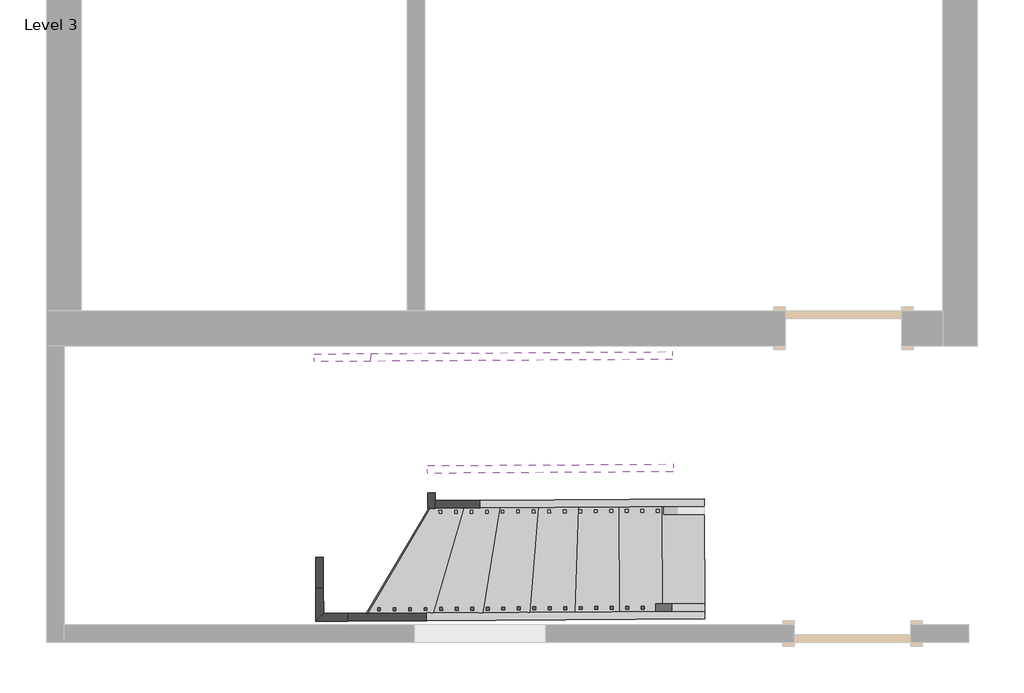
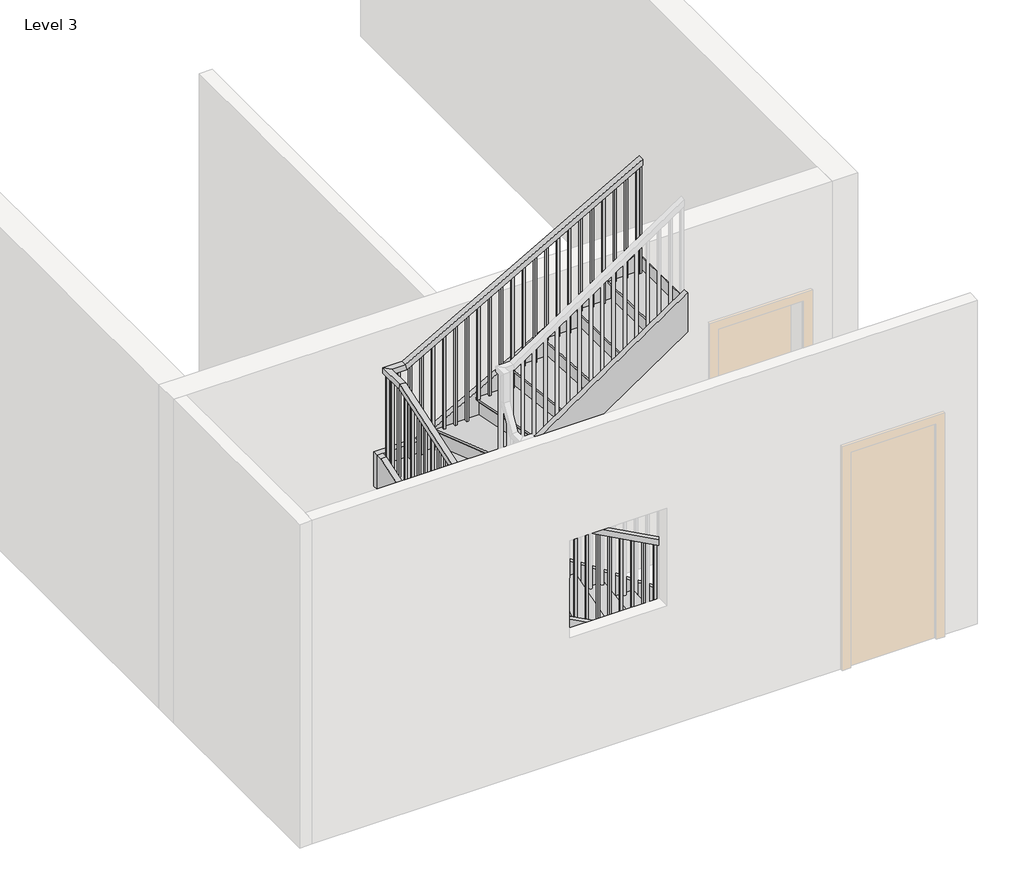
# One storey, part 2 of 2: 9 members, 1 railing, 1 stair flight.
"""IFC4 building model written with IfcOpenShell, lengths in millimetres."""

from ifc_helpers import new_model, si_unit, frame, origin, place, context, project, spatial, polyline, outline, extrude, faceted_brep, transform, mapped, element, save
from components import stair_flight_20cd7bae

model = new_model("IFC4")

# Units and contexts
model_context = context("Model", 3, world=origin())
ifc_project = project(units=[si_unit("LENGTHUNIT", "METRE", prefix="MILLI")], contexts=[model_context])

# Site, building, storey
site = spatial("IfcSite", under=ifc_project)
building = spatial("IfcBuilding", under=site)
storey = spatial("IfcBuildingStorey", under=building, Name="Level 3", Elevation=3200.4)

# Members
placement = place(None, origin())
element("IfcMember", 1, ObjectType="Stringer - 2\" Width", at=placement, inside=storey, context=model_context, shape_type="SweptSolid", body=[
    extrude(outline(polyline([(-106.4787477, -199.0602913), (0.0, 0.0), (2650.4216713, 0.0), (2487.3820108, -304.8), (91.199922, -304.8), (-106.4787477, -199.0602913)])), frame((-116.1777511, -4276.2080688, 3426.1492487), z_axis=(-0.006129891180436153, 0.9999812120405643, 0.0), x_axis=(-0.8817595296628616, -0.005405191516664865, 0.47166822635555733)), (0.0, 0.0, 1.0), 50.8),
])
element("IfcMember", 2, ObjectType="Stringer - 2\" Width", at=placement, inside=storey, context=model_context, shape_type="SweptSolid", body=[
    extrude(outline(polyline([(-2453.5237158, -4239.7350599), (-2453.2123174, -4290.5341055), (-2663.1420684, -4291.8209762), (-2612.6544213, -4240.7105322), (-2453.5237158, -4239.7350599)])), frame((0.0, 0.0, 4330.6029558), z_axis=(0.0, 0.0, 1.0), x_axis=(1.0, 0.0, 0.0)), (0.0, 0.0, 1.0), 345.6659817),
])
element("IfcMember", 3, ObjectType="Stringer - 2\" Width", at=placement, inside=storey, context=model_context, shape_type="SweptSolid", body=[
    extrude(outline(polyline([(-2612.6544213, -4240.7105322), (-2663.1420684, -4291.8209762), (-2664.4731567, -4074.6779247), (-2613.6741111, -4074.3665263), (-2612.6544213, -4240.7105322)])), frame((0.0, 0.0, 4330.6029558), z_axis=(0.0, 0.0, 1.0), x_axis=(1.0, 0.0, 0.0)), (0.0, 0.0, 1.0), 345.6659817),
])
element("IfcMember", 4, ObjectType="Stringer - 2\" Width", at=placement, inside=storey, context=model_context, shape_type="SweptSolid", body=[
    extrude(outline(polyline([(-112.9595567, -326.688092), (0.0, 0.0), (1516.7940002, 1e-07), (1565.1210838, -16.7101466), (1457.9394259, -326.6880919), (-112.9595567, -326.688092)])), frame((-2664.4731567, -4074.6779247, 4676.2689375), z_axis=(0.9999812120405643, 0.006129891180436426, 0.0), x_axis=(-0.005793345483301552, 0.9450798501367781, 0.3267881791215163)), (0.0, 0.0, 1.0), 50.8),
])
element("IfcMember", 5, ObjectType="Stringer - 2\" Width", at=placement, inside=storey, context=model_context, shape_type="SweptSolid", body=[
    extrude(outline(polyline([(-111.800968, -163.7049666), (0.0, 0.0), (2130.8093531, 0.0), (1922.648686, -304.8000001), (94.7979387, -304.8000001), (-111.800968, -163.7049666)])), frame((-120.6930289, -3539.621908, 3398.6391801), z_axis=(-0.006129891180436334, 0.9999812120405644, 0.0), x_axis=(-0.8257797012408891, -0.005062034812924603, 0.5639700885880925)), (0.0, 0.0, 1.0), 50.8),
])
element("IfcMember", 6, ObjectType="Stringer - 2\" Width", at=placement, inside=storey, context=model_context, shape_type="SweptSolid", body=[
    extrude(outline(polyline([(-476.3090819, -288.3824073), (0.0, 0.0), (441.380003, 0.0), (-62.0453256, -304.8), (-466.3690133, -304.8), (-476.3090819, -288.3824073)])), frame((-1931.0711854, -3550.7195376, 4822.7542381), z_axis=(0.9999812120405644, 0.006129891180436036, 0.0), x_axis=(-0.00317479975135555, 0.5179113315223286, 0.8554284150806002)), (0.0, 0.0, 1.0), 50.8),
])
element("IfcMember", 7, ObjectType="Stringer - 2\" Width", at=placement, inside=storey, context=model_context, shape_type="SweptSolid", body=[
    extrude(outline(polyline([(205.0123517, -304.8), (0.0, 0.0), (1938.1040339, 0.0), (2143.1163855, -304.8), (205.0123517, -304.8)])), frame((-1932.4724786, -3322.1238325, 4867.3006308), z_axis=(-0.006129891180436482, 0.9999812120405644, 0.0), x_axis=(0.8297505463599371, 0.005086376118722323, 0.5581112430271987)), (0.0, 0.0, 1.0), 50.8),
])
element("IfcMember", 8, ObjectType="Stringer - 2\" Width", at=placement, inside=storey, context=model_context, shape_type="SweptSolid", body=[
    extrude(outline(polyline([(-2673.5739172, -2590.0529496), (-2673.8853157, -2539.253904), (-2303.2697085, -2536.982028), (-2302.9583101, -2587.7810735), (-2673.5739172, -2590.0529496)])), frame((0.0, 0.0, 4849.4329153), z_axis=(0.0, 0.0, 1.0), x_axis=(1.0, 0.0, 0.0)), (0.0, 0.0, 1.0), 322.5063717),
])
element("IfcMember", 9, ObjectType="Stringer - 2\" Width", at=placement, inside=storey, context=model_context, shape_type="SweptSolid", body=[
    extrude(outline(polyline([(155.3220552, -282.6400873), (0.0, 0.0), (2252.6037587, 1e-07), (2407.9258139, -282.6400872), (155.3220552, -282.6400873)])), frame((-2302.9583101, -2587.7810735, 4849.4329153), z_axis=(-0.00612989118043627, 0.9999812120405644, 0.0), x_axis=(0.8763695910030254, 0.005372151158450033, 0.48160926066378834)), (0.0, 0.0, 1.0), 50.8),
])

# Railing
element("IfcRailing", 10, ObjectType="Handrail - Rectangular", at=placement, inside=storey, context=model_context, shape_type="SolidModel", body=[
    faceted_brep([(-116.4891496, -4225.4090232, 4284.1333333), (-116.4891496, -4225.4090232, 4226.3022634), (-116.800548, -4174.6099776, 4226.3022634), (-116.800548, -4174.6099776, 4284.1333333), (-2474.2717021, -4239.8622452, 5566.8653479), (-2487.1954725, -4239.941468, 5516.0653479), (-2487.506871, -4189.1424224, 5516.0653479), (-2474.5831006, -4189.0631997, 5566.8653479), (-2612.6544213, -4240.7105322, 5566.8653479), (-2612.6544213, -4240.7105322, 5516.0653479), (-2562.1667742, -4189.6000881, 5516.0653479), (-2562.1667742, -4189.6000881, 5566.8653479), (-2613.899826, -4037.5452114, 5566.8653479), (-2613.9521428, -4029.010664, 5516.0653479), (-2563.1530973, -4028.6992655, 5516.0653479), (-2563.1007804, -4037.2338129, 5566.8653479), (-2621.180916, -2849.7666717, 5977.5734867), (-2621.2332328, -2841.2321243, 5926.7734867), (-2570.4341872, -2840.9207258, 5926.7734867), (-2570.3818704, -2849.4552732, 5977.5734867), (-2622.7748716, -2589.7415511, 5977.5734867), (-2622.7748716, -2589.7415511, 5926.7734867), (-2571.6644276, -2640.2291982, 5926.7734867), (-2571.6644276, -2640.2291982, 5977.5734867), (-2452.0429693, -2588.6949634, 5977.5734867), (-2438.8245474, -2588.6139344, 5926.7734867), (-2438.513149, -2639.41298, 5926.7734867), (-2451.7315708, -2639.494009, 5977.5734867), (-328.8448754, -2575.6797456, 7162.8), (-328.533477, -2626.4787912, 7162.8), (-328.533477, -2626.4787912, 7104.62112), (-328.8448754, -2575.6797456, 7104.62112)], [[[0, 1, 2, 3]], [[1, 0, 4, 5]], [[2, 1, 5, 6]], [[3, 2, 6, 7]], [[0, 3, 7, 4]], [[5, 4, 8, 9]], [[6, 5, 9, 10]], [[7, 6, 10, 11]], [[4, 7, 11, 8]], [[9, 8, 12, 13]], [[10, 9, 13, 14]], [[11, 10, 14, 15]], [[8, 11, 15, 12]], [[13, 12, 16, 17]], [[14, 13, 17, 18]], [[15, 14, 18, 19]], [[12, 15, 19, 16]], [[17, 16, 20, 21]], [[18, 17, 21, 22]], [[19, 18, 22, 23]], [[16, 19, 23, 20]], [[21, 20, 24, 25]], [[22, 21, 25, 26]], [[23, 22, 26, 27]], [[20, 23, 27, 24]], [[28, 29, 30, 31]], [[25, 24, 28, 31]], [[26, 25, 31, 30]], [[27, 26, 30, 29]], [[24, 27, 29, 28]]]),
    extrude(outline(polyline([(233.9170124, 19.05), (1235.5250403, 19.05), (1235.5250403, 0.0), (223.2829877, 0.0), (233.9170124, 19.05)])), frame((-352.4784362, -2610.7502757, 7314.591707), z_axis=(-0.0061298911804362555, 0.9999812120405644, 0.0), x_axis=(0.0, 0.0, -1.0)), (0.0, 0.0, 1.0), 19.05),
    extrude(outline(polyline([(233.9170123, 19.05), (1178.8102421, 19.05), (1178.8102421, 0.0), (223.2829877, 0.0), (233.9170123, 19.05)])), frame((-454.0765273, -2611.3730726, 7257.8769088), z_axis=(-0.0061298911804362555, 0.9999812120405644, 0.0), x_axis=(0.0, 0.0, -1.0)), (0.0, 0.0, 1.0), 19.05),
    extrude(outline(polyline([(233.9170124, 19.05), (1122.095444, 19.05), (1122.095444, 0.0), (223.2829877, 0.0), (233.9170124, 19.05)])), frame((-555.6746185, -2611.9958696, 7201.1621107), z_axis=(-0.0061298911804362555, 0.9999812120405644, 0.0), x_axis=(0.0, 0.0, -1.0)), (0.0, 0.0, 1.0), 19.05),
    extrude(outline(polyline([(233.9170123, 19.05), (1234.7139792, 19.05), (1234.7139792, 0.0), (223.2829877, 0.0), (233.9170123, 19.05)])), frame((-657.2727096, -2612.6186665, 7144.4473125), z_axis=(-0.0061298911804362555, 0.9999812120405644, 0.0), x_axis=(0.0, 0.0, -1.0)), (0.0, 0.0, 1.0), 19.05),
    extrude(outline(polyline([(233.9170123, 19.05), (1177.999181, 19.05), (1177.999181, 0.0), (223.2829876, 0.0), (233.9170123, 19.05)])), frame((-758.8708008, -2613.2414635, 7087.7325143), z_axis=(-0.0061298911804362555, 0.9999812120405644, 0.0), x_axis=(0.0, 0.0, -1.0)), (0.0, 0.0, 1.0), 19.05),
    extrude(outline(polyline([(233.9170123, 19.05), (1121.2843829, 19.05), (1121.2843829, 0.0), (223.2829877, 0.0), (233.9170123, 19.05)])), frame((-860.4688919, -2613.8642604, 7031.0177162), z_axis=(-0.0061298911804362555, 0.9999812120405644, 0.0), x_axis=(0.0, 0.0, -1.0)), (0.0, 0.0, 1.0), 19.05),
    extrude(outline(polyline([(233.9170123, 19.0499999), (1233.902918, 19.0499999), (1233.902918, 0.0), (223.2829876, 0.0), (233.9170123, 19.0499999)])), frame((-962.0669831, -2614.4870574, 6974.302918), z_axis=(-0.0061298911804362555, 0.9999812120405644, 0.0), x_axis=(0.0, 0.0, -1.0)), (0.0, 0.0, 1.0), 19.05),
    extrude(outline(polyline([(233.9170123, 19.05), (1177.1881199, 19.05), (1177.1881199, 0.0), (223.2829877, 0.0), (233.9170123, 19.05)])), frame((-1063.6650742, -2615.1098543, 6917.5881199), z_axis=(-0.0061298911804362555, 0.9999812120405644, 0.0), x_axis=(0.0, 0.0, -1.0)), (0.0, 0.0, 1.0), 19.05),
    extrude(outline(polyline([(233.9170123, 19.05), (1120.4733217, 19.05), (1120.4733217, 0.0), (223.2829876, 0.0), (233.9170123, 19.05)])), frame((-1165.2631653, -2615.7326513, 6860.8733217), z_axis=(-0.0061298911804362555, 0.9999812120405644, 0.0), x_axis=(0.0, 0.0, -1.0)), (0.0, 0.0, 1.0), 19.05),
    extrude(outline(polyline([(233.9170123, 19.05), (1233.0918569, 19.05), (1233.0918569, 0.0), (223.2829877, 0.0), (233.9170123, 19.05)])), frame((-1266.8612565, -2616.3554482, 6804.1585236), z_axis=(-0.0061298911804362555, 0.9999812120405644, 0.0), x_axis=(0.0, 0.0, -1.0)), (0.0, 0.0, 1.0), 19.05),
    extrude(outline(polyline([(233.9170123, 19.05), (1176.3770587, 19.05), (1176.3770587, 0.0), (223.2829876, 0.0), (233.9170123, 19.05)])), frame((-1368.4593476, -2616.9782451, 6747.4437254), z_axis=(-0.0061298911804362555, 0.9999812120405644, 0.0), x_axis=(0.0, 0.0, -1.0)), (0.0, 0.0, 1.0), 19.05),
    extrude(outline(polyline([(233.9170123, 19.05), (1288.995594, 19.05), (1288.995594, 0.0), (223.2829877, 0.0), (233.9170123, 19.05)])), frame((-1470.0574388, -2617.6010421, 6690.7289273), z_axis=(-0.0061298911804362555, 0.9999812120405644, 0.0), x_axis=(0.0, 0.0, -1.0)), (0.0, 0.0, 1.0), 19.05),
    extrude(outline(polyline([(233.9170123, 19.05), (1232.2807958, 19.05), (1232.2807958, 0.0), (223.2829876, 0.0), (233.9170123, 19.05)])), frame((-1571.6555299, -2618.223839, 6634.0141291), z_axis=(-0.0061298911804362555, 0.9999812120405644, 0.0), x_axis=(0.0, 0.0, -1.0)), (0.0, 0.0, 1.0), 19.05),
    extrude(outline(polyline([(233.9170123, 19.05), (1175.5659977, 19.05), (1175.5659977, 0.0), (223.2829877, 0.0), (233.9170123, 19.05)])), frame((-1673.2536211, -2618.846636, 6577.299331), z_axis=(-0.0061298911804362555, 0.9999812120405644, 0.0), x_axis=(0.0, 0.0, -1.0)), (0.0, 0.0, 1.0), 19.05),
    extrude(outline(polyline([(233.9170123, 19.05), (1118.8511995, 19.05), (1118.8511995, 0.0), (223.2829876, 0.0), (233.9170123, 19.05)])), frame((-1774.8517122, -2619.4694329, 6520.5845328), z_axis=(-0.0061298911804362555, 0.9999812120405644, 0.0), x_axis=(0.0, 0.0, -1.0)), (0.0, 0.0, 1.0), 19.05),
    extrude(outline(polyline([(233.9170123, 19.05), (1231.4697347, 19.05), (1231.4697347, 0.0), (223.2829877, 0.0), (233.9170123, 19.05)])), frame((-1876.4498033, -2620.0922299, 6463.8697347), z_axis=(-0.0061298911804362555, 0.9999812120405644, 0.0), x_axis=(0.0, 0.0, -1.0)), (0.0, 0.0, 1.0), 19.05),
    extrude(outline(polyline([(233.9170123, 19.05), (1174.7549365, 19.05), (1174.7549365, 0.0), (223.2829876, 0.0), (233.9170123, 19.05)])), frame((-1978.0478945, -2620.7150268, 6407.1549365), z_axis=(-0.0061298911804362555, 0.9999812120405644, 0.0), x_axis=(0.0, 0.0, -1.0)), (0.0, 0.0, 1.0), 19.05),
    extrude(outline(polyline([(233.9170124, 19.05), (1118.0401384, 19.05), (1118.0401384, 0.0), (223.2829877, 0.0), (233.9170124, 19.05)])), frame((-2079.6459856, -2621.3378238, 6350.4401384), z_axis=(-0.0061298911804362555, 0.9999812120405644, 0.0), x_axis=(0.0, 0.0, -1.0)), (0.0, 0.0, 1.0), 19.05),
    extrude(outline(polyline([(233.9170123, 19.05), (1230.6586735, 19.05), (1230.6586735, 0.0), (223.2829876, 0.0), (233.9170123, 19.05)])), frame((-2181.2440768, -2621.9606207, 6293.7253402), z_axis=(-0.0061298911804362555, 0.9999812120405644, 0.0), x_axis=(0.0, 0.0, -1.0)), (0.0, 0.0, 1.0), 19.05),
    extrude(outline(polyline([(233.9170124, 19.05), (1173.9438754, 19.05), (1173.9438754, 0.0), (223.2829877, 0.0), (233.9170124, 19.05)])), frame((-2282.8421679, -2622.5834176, 6237.0105421), z_axis=(-0.0061298911804362555, 0.9999812120405644, 0.0), x_axis=(0.0, 0.0, -1.0)), (0.0, 0.0, 1.0), 19.05),
    extrude(outline(polyline([(233.9170123, 19.05), (1117.2290772, 19.05), (1117.2290772, 0.0), (223.2829877, 0.0), (233.9170123, 19.05)])), frame((-2384.4402591, -2623.2062146, 6180.2957439), z_axis=(-0.0061298911804362555, 0.9999812120405644, 0.0), x_axis=(0.0, 0.0, -1.0)), (0.0, 0.0, 1.0), 19.05),
    extrude(outline(polyline([(-2505.2047667, -2604.8961439), (-2486.1551246, -2604.7793694), (-2486.0383502, -2623.8290115), (-2505.0879923, -2623.945786), (-2505.2047667, -2604.8961439)])), frame((0.0, 0.0, 5063.0666667), z_axis=(0.0, 0.0, 1.0), x_axis=(1.0, 0.0, 0.0)), (0.0, 0.0, 1.0), 863.70682),
    extrude(outline(polyline([(-2606.2189857, -2700.7671513), (-2606.3357602, -2681.7175092), (-2587.2861181, -2681.6007347), (-2587.1693436, -2700.6503768), (-2606.2189857, -2700.7671513)])), frame((0.0, 0.0, 5063.0666667), z_axis=(0.0, 0.0, 1.0), x_axis=(1.0, 0.0, 0.0)), (0.0, 0.0, 1.0), 863.70682),
    extrude(outline(polyline([(-2605.5961888, -2802.3652424), (-2605.7129632, -2783.3156003), (-2586.6633211, -2783.1988259), (-2586.5465467, -2802.248468), (-2605.5961888, -2802.3652424)])), frame((0.0, 0.0, 5063.0666667), z_axis=(0.0, 0.0, 1.0), x_axis=(1.0, 0.0, 0.0)), (0.0, 0.0, 1.0), 863.70682),
    extrude(outline(polyline([(225.3065228, 19.0499999), (1243.2088863, 19.0499999), (1243.2088863, 0.0), (231.8934772, 0.0), (225.3065228, 19.0499999)])), frame((-2604.9733918, -2903.9633335, 6136.9422196), z_axis=(0.9999812120405643, 0.0061298911804362685, 0.0), x_axis=(0.0, 0.0, -1.0)), (0.0, 0.0, 1.0), 19.05),
    extrude(outline(polyline([(225.3065229, 19.05), (1208.078463, 19.05), (1208.078463, 0.0), (231.8934772, 0.0), (225.3065229, 19.05)])), frame((-2604.3505949, -3005.5614247, 6101.8117963), z_axis=(0.9999812120405643, 0.0061298911804362685, 0.0), x_axis=(0.0, 0.0, -1.0)), (0.0, 0.0, 1.0), 19.05),
    extrude(outline(polyline([(225.3065228, 19.05), (1172.9480396, 19.05), (1172.9480396, 0.0), (231.8934772, 0.0), (225.3065228, 19.05)])), frame((-2603.727798, -3107.1595158, 6066.6813729), z_axis=(0.9999812120405643, 0.0061298911804362685, 0.0), x_axis=(0.0, 0.0, -1.0)), (0.0, 0.0, 1.0), 19.05),
    extrude(outline(polyline([(225.3065228, 19.05), (1137.8176163, 19.05), (1137.8176163, 0.0), (231.8934772, 0.0), (225.3065228, 19.05)])), frame((-2603.105001, -3208.757607, 6031.5509496), z_axis=(0.9999812120405643, 0.0061298911804362685, 0.0), x_axis=(0.0, 0.0, -1.0)), (0.0, 0.0, 1.0), 19.05),
    extrude(outline(polyline([(225.3065228, 19.05), (1102.687193, 19.05), (1102.687193, 0.0), (231.8934772, 0.0), (225.3065228, 19.05)])), frame((-2602.4822041, -3310.3556981, 5996.4205263), z_axis=(0.9999812120405643, 0.0061298911804362685, 0.0), x_axis=(0.0, 0.0, -1.0)), (0.0, 0.0, 1.0), 19.05),
    extrude(outline(polyline([(225.3065228, 19.05), (1236.890103, 19.05), (1236.890103, 0.0), (231.8934772, 0.0), (225.3065228, 19.05)])), frame((-2601.8594071, -3411.9537893, 5961.290103), z_axis=(0.9999812120405643, 0.0061298911804362685, 0.0), x_axis=(0.0, 0.0, -1.0)), (0.0, 0.0, 1.0), 19.05),
    extrude(outline(polyline([(225.3065229, 19.05), (1201.7596797, 19.05), (1201.7596797, 0.0), (231.8934772, 0.0), (225.3065229, 19.05)])), frame((-2601.2366102, -3513.5518804, 5926.1596797), z_axis=(0.9999812120405643, 0.0061298911804362685, 0.0), x_axis=(0.0, 0.0, -1.0)), (0.0, 0.0, 1.0), 19.05),
    extrude(outline(polyline([(225.3065228, 19.0499999), (1166.6292563, 19.0499999), (1166.6292563, 0.0), (231.8934772, 0.0), (225.3065228, 19.0499999)])), frame((-2600.6138132, -3615.1499715, 5891.0292563), z_axis=(0.9999812120405643, 0.0061298911804362685, 0.0), x_axis=(0.0, 0.0, -1.0)), (0.0, 0.0, 1.0), 19.05),
    extrude(outline(polyline([(225.3065228, 19.05), (1131.498833, 19.05), (1131.498833, 0.0), (231.8934772, 0.0), (225.3065228, 19.05)])), frame((-2599.9910163, -3716.7480627, 5855.898833), z_axis=(0.9999812120405643, 0.0061298911804362685, 0.0), x_axis=(0.0, 0.0, -1.0)), (0.0, 0.0, 1.0), 19.05),
    extrude(outline(polyline([(225.3065228, 19.05), (1096.3684097, 19.05), (1096.3684097, 0.0), (231.8934772, 0.0), (225.3065228, 19.05)])), frame((-2599.3682194, -3818.3461538, 5820.7684097), z_axis=(0.9999812120405643, 0.0061298911804362685, 0.0), x_axis=(0.0, 0.0, -1.0)), (0.0, 0.0, 1.0), 19.05),
    extrude(outline(polyline([(225.3065228, 19.05), (1230.5713197, 19.05), (1230.5713197, 0.0), (231.8934772, 0.0), (225.3065228, 19.05)])), frame((-2598.7454224, -3919.944245, 5785.6379864), z_axis=(0.9999812120405643, 0.0061298911804362685, 0.0), x_axis=(0.0, 0.0, -1.0)), (0.0, 0.0, 1.0), 19.05),
    extrude(outline(polyline([(225.3065228, 19.05), (1195.4408963, 19.05), (1195.4408963, 0.0), (231.8934771, 0.0), (225.3065228, 19.05)])), frame((-2598.1226255, -4021.5423361, 5750.507563), z_axis=(0.9999812120405643, 0.0061298911804362685, 0.0), x_axis=(0.0, 0.0, -1.0)), (0.0, 0.0, 1.0), 19.05),
    extrude(outline(polyline([(-2597.4998285, -4123.1404273), (-2597.6166029, -4104.0907852), (-2578.5669609, -4103.9740107), (-2578.4501864, -4123.0236528), (-2597.4998285, -4123.1404273)])), frame((0.0, 0.0, 4555.0666667), z_axis=(0.0, 0.0, 1.0), x_axis=(1.0, 0.0, 0.0)), (0.0, 0.0, 1.0), 960.9986813),
    extrude(outline(polyline([(-2545.415828, -4224.4230609), (-2564.4654701, -4224.5398353), (-2564.5822445, -4205.4901932), (-2545.5326024, -4205.3734188), (-2545.415828, -4224.4230609)])), frame((0.0, 0.0, 4555.0666667), z_axis=(0.0, 0.0, 1.0), x_axis=(1.0, 0.0, 0.0)), (0.0, 0.0, 1.0), 960.9986813),
    extrude(outline(polyline([(223.4181002, 19.05), (1171.1283424, 19.05), (1171.1283424, 0.0), (233.7818998, 0.0), (223.4181002, 19.05)])), frame((-2443.8177368, -4223.800264, 5726.1950091), z_axis=(-0.006129891180436165, 0.9999812120405643, 0.0), x_axis=(0.0, 0.0, -1.0)), (0.0, 0.0, 1.0), 19.05),
    extrude(outline(polyline([(223.4181002, 19.05), (1115.8547448, 19.05), (1115.8547448, 0.0), (233.7818998, 0.0), (223.4181002, 19.05)])), frame((-2342.2196457, -4223.177467, 5670.9214115), z_axis=(-0.006129891180436165, 0.9999812120405643, 0.0), x_axis=(0.0, 0.0, -1.0)), (0.0, 0.0, 1.0), 19.05),
    extrude(outline(polyline([(223.4181002, 19.05), (1229.9144805, 19.05), (1229.9144805, 0.0), (233.7818997, 0.0), (223.4181002, 19.05)])), frame((-2240.6215545, -4222.5546701, 5615.6478138), z_axis=(-0.006129891180436165, 0.9999812120405643, 0.0), x_axis=(0.0, 0.0, -1.0)), (0.0, 0.0, 1.0), 19.05),
    extrude(outline(polyline([(223.4181002, 19.05), (1174.6408829, 19.05), (1174.6408829, 0.0), (233.7818998, 0.0), (223.4181002, 19.05)])), frame((-2139.0234634, -4221.9318731, 5560.3742162), z_axis=(-0.006129891180436165, 0.9999812120405643, 0.0), x_axis=(0.0, 0.0, -1.0)), (0.0, 0.0, 1.0), 19.05),
    extrude(outline(polyline([(223.4181003, 19.0499999), (1119.3672853, 19.0499999), (1119.3672853, 0.0), (233.7818998, 0.0), (223.4181003, 19.0499999)])), frame((-2037.4253723, -4221.3090762, 5505.1006186), z_axis=(-0.006129891180436165, 0.9999812120405643, 0.0), x_axis=(0.0, 0.0, -1.0)), (0.0, 0.0, 1.0), 19.05),
    extrude(outline(polyline([(223.4181002, 19.05), (1064.0936876, 19.05), (1064.0936876, 0.0), (233.7818998, 0.0), (223.4181002, 19.05)])), frame((-1935.8272811, -4220.6862792, 5449.8270209), z_axis=(-0.006129891180436165, 0.9999812120405643, 0.0), x_axis=(0.0, 0.0, -1.0)), (0.0, 0.0, 1.0), 19.05),
    extrude(outline(polyline([(223.4181002, 19.05), (1178.1534233, 19.05), (1178.1534233, 0.0), (233.7818998, 0.0), (223.4181002, 19.05)])), frame((-1834.22919, -4220.0634823, 5394.5534233), z_axis=(-0.006129891180436165, 0.9999812120405643, 0.0), x_axis=(0.0, 0.0, -1.0)), (0.0, 0.0, 1.0), 19.05),
    extrude(outline(polyline([(223.4181002, 19.05), (1122.8798256, 19.05), (1122.8798256, 0.0), (233.7818997, 0.0), (223.4181002, 19.05)])), frame((-1732.6310988, -4219.4406854, 5339.2798256), z_axis=(-0.006129891180436165, 0.9999812120405643, 0.0), x_axis=(0.0, 0.0, -1.0)), (0.0, 0.0, 1.0), 19.05),
    extrude(outline(polyline([(223.4181002, 19.05), (1067.606228, 19.05), (1067.606228, 0.0), (233.7818998, 0.0), (223.4181002, 19.05)])), frame((-1631.0330077, -4218.8178884, 5284.006228), z_axis=(-0.006129891180436165, 0.9999812120405643, 0.0), x_axis=(0.0, 0.0, -1.0)), (0.0, 0.0, 1.0), 19.05),
    extrude(outline(polyline([(223.4181003, 19.05), (1181.6659637, 19.05), (1181.6659637, 0.0), (233.7818998, 0.0), (223.4181003, 19.05)])), frame((-1529.4349165, -4218.1950915, 5228.7326304), z_axis=(-0.006129891180436165, 0.9999812120405643, 0.0), x_axis=(0.0, 0.0, -1.0)), (0.0, 0.0, 1.0), 19.05),
    extrude(outline(polyline([(223.4181002, 19.05), (1126.392366, 19.05), (1126.392366, 0.0), (233.7818998, 0.0), (223.4181002, 19.05)])), frame((-1427.8368254, -4217.5722945, 5173.4590327), z_axis=(-0.006129891180436165, 0.9999812120405643, 0.0), x_axis=(0.0, 0.0, -1.0)), (0.0, 0.0, 1.0), 19.05),
    extrude(outline(polyline([(223.4181002, 19.0499999), (1071.1187684, 19.0499999), (1071.1187684, 0.0), (233.7818998, 0.0), (223.4181002, 19.0499999)])), frame((-1326.2387343, -4216.9494976, 5118.1854351), z_axis=(-0.006129891180436165, 0.9999812120405643, 0.0), x_axis=(0.0, 0.0, -1.0)), (0.0, 0.0, 1.0), 19.05),
    extrude(outline(polyline([(223.4181002, 19.05), (1185.1785041, 19.05), (1185.1785041, 0.0), (233.7818997, 0.0), (223.4181002, 19.05)])), frame((-1224.6406431, -4216.3267006, 5062.9118374), z_axis=(-0.006129891180436165, 0.9999812120405643, 0.0), x_axis=(0.0, 0.0, -1.0)), (0.0, 0.0, 1.0), 19.05),
    extrude(outline(polyline([(223.4181002, 19.05), (1129.9049065, 19.05), (1129.9049065, 0.0), (233.7818998, 0.0), (223.4181002, 19.05)])), frame((-1123.042552, -4215.7039037, 5007.6382398), z_axis=(-0.006129891180436165, 0.9999812120405643, 0.0), x_axis=(0.0, 0.0, -1.0)), (0.0, 0.0, 1.0), 19.05),
    extrude(outline(polyline([(223.4181003, 19.05), (1074.6313089, 19.05), (1074.6313089, 0.0), (233.7818998, 0.0), (223.4181003, 19.05)])), frame((-1021.4444608, -4215.0811067, 4952.3646422), z_axis=(-0.006129891180436165, 0.9999812120405643, 0.0), x_axis=(0.0, 0.0, -1.0)), (0.0, 0.0, 1.0), 19.05),
    extrude(outline(polyline([(223.4181002, 19.05), (1188.6910445, 19.05), (1188.6910445, 0.0), (233.7818998, 0.0), (223.4181002, 19.05)])), frame((-919.8463697, -4214.4583098, 4897.0910445), z_axis=(-0.006129891180436165, 0.9999812120405643, 0.0), x_axis=(0.0, 0.0, -1.0)), (0.0, 0.0, 1.0), 19.05),
    extrude(outline(polyline([(223.4181002, 19.05), (1133.4174469, 19.05), (1133.4174469, 0.0), (233.7818998, 0.0), (223.4181002, 19.05)])), frame((-818.2482785, -4213.8355129, 4841.8174469), z_axis=(-0.006129891180436165, 0.9999812120405643, 0.0), x_axis=(0.0, 0.0, -1.0)), (0.0, 0.0, 1.0), 19.05),
    extrude(outline(polyline([(223.4181002, 19.05), (1078.1438492, 19.05), (1078.1438492, 0.0), (233.7818997, 0.0), (223.4181002, 19.05)])), frame((-716.6501874, -4213.2127159, 4786.5438492), z_axis=(-0.006129891180436165, 0.9999812120405643, 0.0), x_axis=(0.0, 0.0, -1.0)), (0.0, 0.0, 1.0), 19.05),
    extrude(outline(polyline([(223.4181002, 19.0499999), (1192.2035849, 19.0499999), (1192.2035849, 0.0), (233.7818998, 0.0), (223.4181002, 19.0499999)])), frame((-615.0520963, -4212.589919, 4731.2702516), z_axis=(-0.006129891180436165, 0.9999812120405643, 0.0), x_axis=(0.0, 0.0, -1.0)), (0.0, 0.0, 1.0), 19.05),
    extrude(outline(polyline([(223.4181003, 19.05), (1136.9299873, 19.05), (1136.9299873, 0.0), (233.7818998, 0.0), (223.4181003, 19.05)])), frame((-513.4540051, -4211.967122, 4675.996654), z_axis=(-0.006129891180436165, 0.9999812120405643, 0.0), x_axis=(0.0, 0.0, -1.0)), (0.0, 0.0, 1.0), 19.05),
    extrude(outline(polyline([(223.4181002, 19.05), (1081.6563896, 19.05), (1081.6563896, 0.0), (233.7818998, 0.0), (223.4181002, 19.05)])), frame((-411.855914, -4211.3443251, 4620.7230563), z_axis=(-0.006129891180436165, 0.9999812120405643, 0.0), x_axis=(0.0, 0.0, -1.0)), (0.0, 0.0, 1.0), 19.05),
    extrude(outline(polyline([(223.4181002, 19.05), (1195.7161254, 19.05), (1195.7161254, 0.0), (233.7818998, 0.0), (223.4181002, 19.05)])), frame((-310.2578228, -4210.7215281, 4565.4494587), z_axis=(-0.006129891180436165, 0.9999812120405643, 0.0), x_axis=(0.0, 0.0, -1.0)), (0.0, 0.0, 1.0), 19.05),
    extrude(outline(polyline([(223.4181002, 19.05), (1140.4425277, 19.05), (1140.4425277, 0.0), (233.7818997, 0.0), (223.4181002, 19.05)])), frame((-208.6597317, -4210.0987312, 4510.175861), z_axis=(-0.006129891180436165, 0.9999812120405643, 0.0), x_axis=(0.0, 0.0, -1.0)), (0.0, 0.0, 1.0), 19.05),
    extrude(outline(polyline([(-2606.6860834, -2624.5685829), (-2606.8028579, -2605.5189408), (-2587.7532158, -2605.4021664), (-2587.6364414, -2624.4518085), (-2606.6860834, -2624.5685829)])), frame((0.0, 0.0, 5063.0666667), z_axis=(0.0, 0.0, 1.0), x_axis=(1.0, 0.0, 0.0)), (0.0, 0.0, 1.0), 863.70682),
    extrude(outline(polyline([(-2577.8273895, -4224.621744), (-2596.8770316, -4224.7385184), (-2596.993806, -4205.6888763), (-2577.9441639, -4205.5721019), (-2577.8273895, -4224.621744)])), frame((0.0, 0.0, 4555.0666667), z_axis=(0.0, 0.0, 1.0), x_axis=(1.0, 0.0, 0.0)), (0.0, 0.0, 1.0), 960.9986813),
    extrude(outline(polyline([(233.9170123, 19.05), (1248.8374409, 19.05), (1248.8374409, 0.0), (223.2829876, 0.0), (233.9170123, 19.05)])), frame((-328.630789, -2610.6040895, 7327.9041076), z_axis=(-0.0061298911804362555, 0.9999812120405644, 0.0), x_axis=(0.0, 0.0, -1.0)), (0.0, 0.0, 1.0), 19.05),
    extrude(outline(polyline([(223.4181002, 19.05), (1090.3508299, 19.05), (1090.3508299, 0.0), (233.7818998, 0.0), (223.4181002, 19.05)])), frame((-116.5864616, -4209.5343215, 4460.0841632), z_axis=(-0.006129891180436165, 0.9999812120405643, 0.0), x_axis=(0.0, 0.0, -1.0)), (0.0, 0.0, 1.0), 19.05),
])

# Stair flight
stair_flight_shape = stair_flight_20cd7bae(model_context)
element("IfcStairFlight", 11, ObjectType="2\" Tread 1\" Nosing 1/4\" Riser", at=placement, inside=storey, context=model_context, shape_type="MappedRepresentation", body=[
    mapped(stair_flight_shape, transform((0.0, 0.0, 0.0), x_axis=(1.0, 0.0, 0.0), y_axis=(0.0, 1.0, 0.0), z_axis=(0.0, 0.0, 1.0))),
])

save(model, "model.ifc")

# Revit data of these elements
# Type "Handrail - Rectangular"
#   Assembly Code = "C2010400"
#   built-in parameter 1008612 = 0.0416667 (stored number, unit not read)
#   built-in parameter 1008611 = 0.0416667 (stored number, unit not read)
#   built-in parameter 1008609 = 0.333333 (stored number, unit not read)
#   built-in parameter 1008604 = 0.166667 (stored number, unit not read)
#   built-in parameter 1008603 = 0.166667 (stored number, unit not read)
#   Railing Height = 3' - 0"
#   built-in parameter 1008630 = 2
#   built-in parameter 1008610 = 2
#   built-in parameter 1008618 = Baluster - Square : 3/4"
# Elements 1, 2, 3, 4, 5, 6, 7, 8, 9 (IfcMember, "Stringer - 2\" Width")
#   Phase Created = New Construction
# Element 10 (IfcRailing, "Handrail - Rectangular")
#   Phase Created = New Construction
# Element 11 (IfcStairFlight, "2\" Tread 1\" Nosing 1/4\" Riser")
#   Phase Created = New Construction
